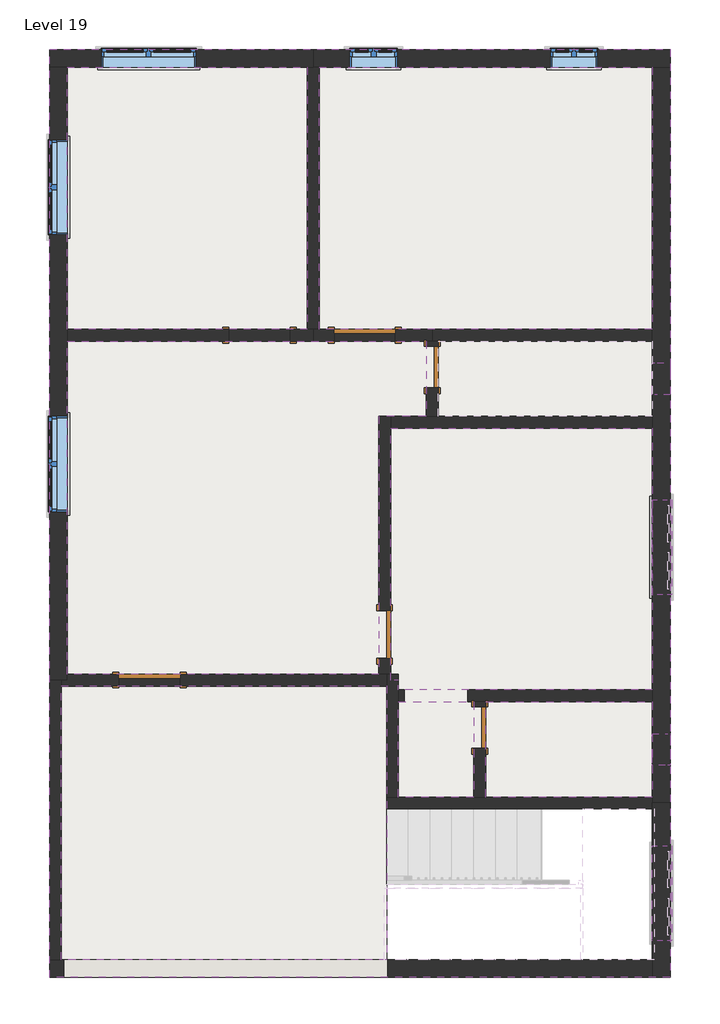
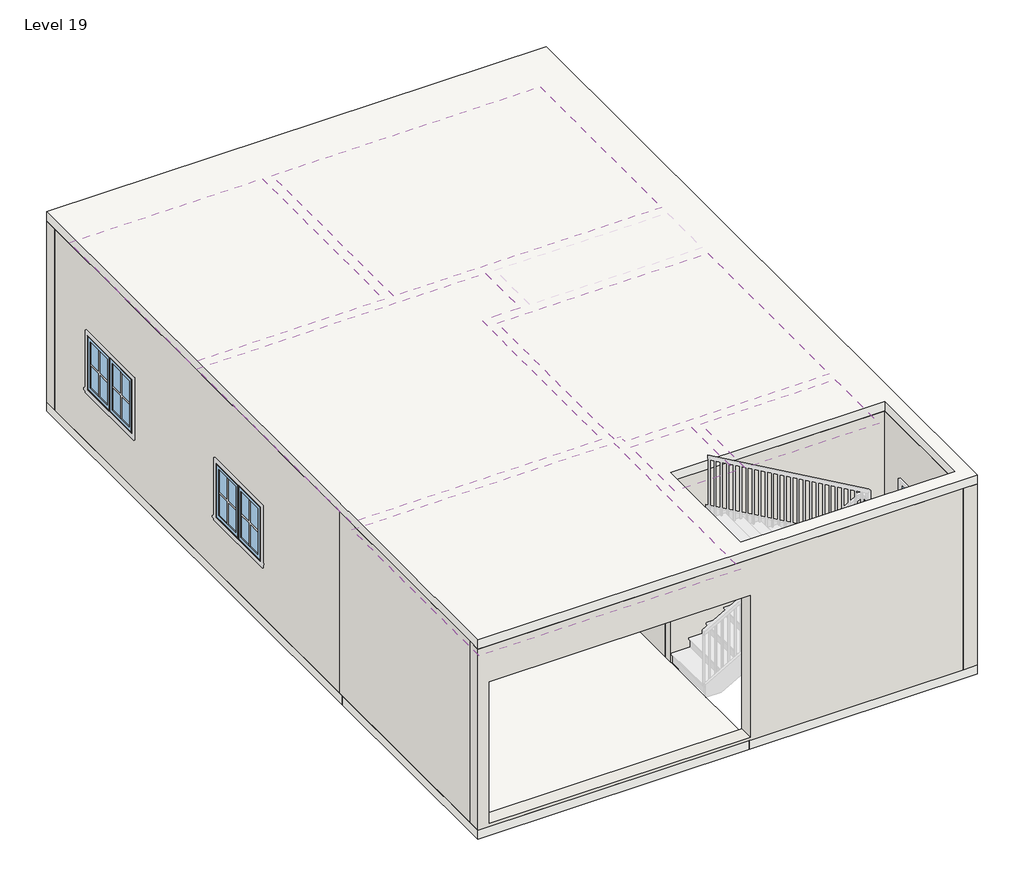
# One storey, part 1 of 2: 27 walls, 13 windows, 7 coverings, 6 doors, 3 slabs.
"""IFC4 building model written with IfcOpenShell, lengths in millimetres."""

from ifc_helpers import new_model, si_unit, frame, origin, place, context, project, spatial, polyline, outline, extrude, faceted_brep, transform, mapped, element, save
from components import door_2908be75, door_9ea4ff49, door_dc34e247, door_b804d09e, fixed_2_415b3208, window_casement_double_3_c417fced, window_casement_double_4_c19c33cb

model = new_model("IFC4")

# Units and contexts
model_context = context("Model", 3, world=origin())
ifc_project = project(units=[si_unit("LENGTHUNIT", "METRE", prefix="MILLI")], contexts=[model_context])

# Site, building, storey
site = spatial("IfcSite", under=ifc_project)
building = spatial("IfcBuilding", under=site)
storey = spatial("IfcBuildingStorey", under=building, Name="Level 19", Elevation=12801.6)

# Coverings
placement = place(None, origin())
element("IfcCovering", 1, ObjectType="2' x 4' ACT System", at=placement, inside=storey, context=model_context, shape_type="SweptSolid", body=[
    extrude(outline(polyline([(-5680.5154463, 2323.8455275), (-5680.5154463, 5678.2330275), (-2607.1154463, 5678.2330275), (-2607.1154463, 2323.8455275), (-5680.5154463, 2323.8455275)])), frame((0.0, 0.0, 15544.8), z_axis=(0.0, 0.0, 1.0), x_axis=(1.0, 0.0, 0.0)), (0.0, 0.0, 1.0), 57.15),
])
element("IfcCovering", 2, ObjectType="2' x 4' ACT System", at=placement, inside=storey, context=model_context, shape_type="SweptSolid", body=[
    extrude(outline(polyline([(-2454.7154463, 2323.8455275), (-2454.7154463, 5678.2330275), (1812.4845537, 5678.2330275), (1812.4845537, 2323.8455275), (-2454.7154463, 2323.8455275)])), frame((0.0, 0.0, 15544.8), z_axis=(0.0, 0.0, 1.0), x_axis=(1.0, 0.0, 0.0)), (0.0, 0.0, 1.0), 57.15),
])
element("IfcCovering", 3, ObjectType="2' x 4' ACT System", at=placement, inside=storey, context=model_context, shape_type="SweptSolid", body=[
    extrude(outline(polyline([(-5680.5154463, -2095.7544725), (-5680.5154463, 2171.4455275), (-1083.1154463, 2171.4455275), (-1083.1154463, 1206.2455275), (-1692.7154463, 1206.2455275), (-1692.7154463, -2095.7544725), (-5680.5154463, -2095.7544725)])), frame((0.0, 0.0, 15544.8), z_axis=(0.0, 0.0, 1.0), x_axis=(1.0, 0.0, 0.0)), (0.0, 0.0, 1.0), 57.15),
])
element("IfcCovering", 4, ObjectType="2' x 4' ACT System", at=placement, inside=storey, context=model_context, shape_type="SweptSolid", body=[
    extrude(outline(polyline([(1812.4845537, 1053.8455275), (1812.4845537, -2298.9544725), (-1438.7154463, -2298.9544725), (-1438.7154463, -2171.9544725), (-1540.3154463, -2171.9544725), (-1540.3154463, 1053.8455275), (1812.4845537, 1053.8455275)])), frame((0.0, 0.0, 15544.8), z_axis=(0.0, 0.0, 1.0), x_axis=(1.0, 0.0, 0.0)), (0.0, 0.0, 1.0), 57.15),
])
element("IfcCovering", 5, ObjectType="2' x 4' ACT System", at=placement, inside=storey, context=model_context, shape_type="SweptSolid", body=[
    extrude(outline(polyline([(1812.4845537, -2451.3544725), (1812.4845537, -3670.5544725), (-321.1154463, -3670.5544725), (-321.1154463, -2451.3544725), (1812.4845537, -2451.3544725)])), frame((0.0, 0.0, 15544.8), z_axis=(0.0, 0.0, 1.0), x_axis=(1.0, 0.0, 0.0)), (0.0, 0.0, 1.0), 57.15),
])
element("IfcCovering", 6, ObjectType="2' x 4' ACT System", at=placement, inside=storey, context=model_context, shape_type="SweptSolid", body=[
    extrude(outline(polyline([(-473.5154463, -2451.3544725), (-473.5154463, -3670.5544725), (-1438.7154463, -3670.5544725), (-1438.7154463, -2451.3544725), (-473.5154463, -2451.3544725)])), frame((0.0, 0.0, 15544.8), z_axis=(0.0, 0.0, 1.0), x_axis=(1.0, 0.0, 0.0)), (0.0, 0.0, 1.0), 57.15),
])
element("IfcCovering", 7, ObjectType="2' x 4' ACT System", at=placement, inside=storey, context=model_context, shape_type="SweptSolid", body=[
    extrude(outline(polyline([(-1591.1154463, -2248.1544725), (-1591.1154463, -5753.3544725), (-5756.7154463, -5753.3544725), (-5756.7154463, -2248.1544725), (-1591.1154463, -2248.1544725)])), frame((0.0, 0.0, 15544.8), z_axis=(0.0, 0.0, 1.0), x_axis=(1.0, 0.0, 0.0)), (0.0, 0.0, 1.0), 57.15),
])

# Doors
door_shape = door_2908be75(model_context)
element("IfcDoor", 8, ObjectType="Single-Flush : 1' 9\"", at=placement, inside=storey, context=model_context, shape_type="MappedRepresentation", body=[
    mapped(door_shape, transform((-397.3154463, -2781.5544725, 12801.6), x_axis=(0.0, 1.0, 0.0), y_axis=(-1.0, 0.0, 0.0), z_axis=(0.0, 0.0, 1.0))),
])
element("IfcDoor", 9, ObjectType="Single-Flush : 1' 9\"", at=placement, inside=storey, context=model_context, shape_type="MappedRepresentation", body=[
    mapped(door_shape, transform((-1006.9154463, 1841.2455275, 12801.6), x_axis=(0.0, 1.0, 0.0), y_axis=(-1.0, 0.0, 0.0), z_axis=(0.0, 0.0, 1.0))),
])
door_2_shape = door_9ea4ff49(model_context)
element("IfcDoor", 10, ObjectType="Single-Flush : 2'0\"", at=placement, inside=storey, context=model_context, shape_type="MappedRepresentation", body=[
    mapped(door_2_shape, transform((-1616.5154463, -1587.7544725, 12801.6), x_axis=(0.0, -1.0, 0.0), y_axis=(1.0, 0.0, 0.0), z_axis=(0.0, 0.0, 1.0))),
])
door_3_shape = door_dc34e247(model_context)
element("IfcDoor", 11, ObjectType="Single-Flush : 2'7\"", at=placement, inside=storey, context=model_context, shape_type="MappedRepresentation", body=[
    mapped(door_3_shape, transform((-4626.4154463, -2171.9544725, 12801.6), x_axis=(-1.0, 0.0, 0.0), y_axis=(0.0, -1.0, 0.0), z_axis=(0.0, 0.0, 1.0))),
])
element("IfcDoor", 12, ObjectType="Single-Flush : 2'7\"", at=placement, inside=storey, context=model_context, shape_type="MappedRepresentation", body=[
    mapped(door_3_shape, transform((-1870.5154463, 2247.6455275, 12801.6), x_axis=(-1.0, 0.0, 0.0), y_axis=(0.0, -1.0, 0.0), z_axis=(0.0, 0.0, 1.0))),
])
door_4_shape = door_b804d09e(model_context)
element("IfcDoor", 13, ObjectType="Single-Flush : 2'7\"", at=placement, inside=storey, context=model_context, shape_type="MappedRepresentation", body=[
    mapped(door_4_shape, transform((-3216.7154463, 2247.6455275, 12801.6), x_axis=(1.0, 0.0, 0.0), y_axis=(0.0, 1.0, 0.0), z_axis=(0.0, 0.0, 1.0))),
])

# Slabs
element("IfcSlab", 14, ObjectType="Generic - 6\"", at=placement, inside=storey, context=model_context, shape_type="SweptSolid", body=[
    extrude(outline(polyline([(-5909.1154463, -2248.1544725), (-5909.1154463, 5906.8330275), (2041.0845537, 5906.8330275), (2041.0845537, -5981.9544725), (-1591.1154463, -5981.9544725), (-1591.1154463, -5753.3544725), (1812.4845537, -5753.3544725), (1812.4845537, -3822.9544725), (-1591.1154463, -3822.9544725), (-1591.1154463, -2248.1544725), (-5756.7154463, -2248.1544725), (-5909.1154463, -2248.1544725)])), frame((0.0, 0.0, 12649.2), z_axis=(0.0, 0.0, 1.0), x_axis=(1.0, 0.0, 0.0)), (0.0, 0.0, 1.0), 152.4),
])
element("IfcSlab", 15, ObjectType="Generic - 6\"", at=placement, inside=storey, context=model_context, shape_type="SweptSolid", body=[
    extrude(outline(polyline([(-1591.1154463, -2248.1544725), (-1591.1154463, -5981.9544725), (-5909.1154463, -5981.9544725), (-5909.1154463, -2248.1544725), (-1591.1154463, -2248.1544725)])), frame((0.0, 0.0, 12649.2), z_axis=(0.0, 0.0, 1.0), x_axis=(1.0, 0.0, 0.0)), (0.0, 0.0, 1.0), 152.4),
])
element("IfcSlab", 16, ObjectType="Generic - 6\"", at=placement, inside=storey, context=model_context, shape_type="SweptSolid", body=[
    extrude(outline(polyline([(2041.0845537, 5906.8330275), (2041.0845537, -5981.9544725), (-5909.1154463, -5981.9544725), (-5909.1154463, 5906.8330275), (2041.0845537, 5906.8330275)]), holes=[polyline([(1812.4845537, -3822.9544725), (-1591.1154463, -3822.9544725), (-1591.1154463, -5753.3544725), (1812.4845537, -5753.3544725), (1812.4845537, -3822.9544725)])]), frame((0.0, 0.0, 15849.6), z_axis=(0.0, 0.0, 1.0), x_axis=(1.0, 0.0, 0.0)), (0.0, 0.0, 1.0), 152.4),
])

# Walls
element("IfcWall", 17, ObjectType="Generic - 6\"", at=placement, inside=storey, context=model_context, shape_type="Brep", body=[
    faceted_brep([(-5909.1154463, -2171.9544725, 12801.6), (-5909.1154463, -5753.3544725, 12801.6), (-5909.1154463, -5753.3544725, 15849.6), (-5909.1154463, -2171.9544725, 15849.6), (-5756.7154463, -2171.9544725, 12801.6), (-5756.7154463, -2171.9544725, 15849.6), (-5756.7154463, -2248.1544725, 15849.6), (-5756.7154463, -5753.3544725, 15849.6), (-5756.7154463, -5753.3544725, 12801.6), (-5756.7154463, -2248.1544725, 12801.6)], [[[0, 1, 2, 3]], [[4, 5, 6, 7, 8, 9]], [[1, 0, 4, 9, 8]], [[3, 2, 7, 6, 5]], [[0, 3, 5, 4]], [[2, 1, 8, 7]]]),
])
element("IfcWall", 18, ObjectType="Generic - 6\"", at=placement, inside=storey, context=model_context, shape_type="Brep", body=[
    faceted_brep([(1812.4845537, -3670.5544725, 12801.6), (-321.1154463, -3670.5544725, 12801.6), (-473.5154463, -3670.5544725, 12801.6), (-1438.7154463, -3670.5544725, 12801.6), (-1591.1154463, -3670.5544725, 12801.6), (-1591.1154463, -3670.5544725, 15849.6), (-1438.7154463, -3670.5544725, 15849.6), (-473.5154463, -3670.5544725, 15849.6), (-321.1154463, -3670.5544725, 15849.6), (1812.4845537, -3670.5544725, 15849.6), (1812.4845537, -3822.9544725, 12801.6), (1812.4845537, -3822.9544725, 15849.6), (-1591.1154463, -3822.9544725, 15849.6), (-1591.1154463, -3822.9544725, 12801.6), (1812.4845537, -3746.7544725, 12801.6), (1812.4845537, -3746.7544725, 15849.6)], [[[0, 1, 2, 3, 4, 5, 6, 7, 8, 9]], [[10, 11, 12, 13]], [[4, 3, 2, 1, 0, 14, 10, 13]], [[9, 8, 7, 6, 5, 12, 11, 15]], [[5, 4, 13, 12]], [[0, 9, 15, 11, 10, 14]]]),
])
element("IfcWall", 19, ObjectType="Generic - 6\"", at=placement, inside=storey, context=model_context, shape_type="Brep", body=[
    faceted_brep([(-1438.7154463, -3670.5544725, 12801.6), (-1438.7154463, -2451.3544725, 12801.6), (-1438.7154463, -2298.9544725, 12801.6), (-1438.7154463, -2095.7544725, 12801.6), (-1438.7154463, -2095.7544725, 15849.6), (-1438.7154463, -2298.9544725, 15849.6), (-1438.7154463, -2451.3544725, 15849.6), (-1438.7154463, -3670.5544725, 15849.6), (-1591.1154463, -3670.5544725, 12801.6), (-1591.1154463, -3670.5544725, 15849.6), (-1591.1154463, -2248.1544725, 15849.6), (-1591.1154463, -2171.9544725, 15849.6), (-1591.1154463, -2095.7544725, 15849.6), (-1591.1154463, -2095.7544725, 12801.6), (-1591.1154463, -2171.9544725, 12801.6), (-1591.1154463, -2248.1544725, 12801.6), (-1540.3154463, -2095.7544725, 12801.6), (-1540.3154463, -2095.7544725, 15849.6)], [[[0, 1, 2, 3, 4, 5, 6, 7]], [[8, 9, 10, 11, 12, 13, 14, 15]], [[3, 2, 1, 0, 8, 15, 14, 13, 16]], [[7, 6, 5, 4, 17, 12, 11, 10, 9]], [[0, 7, 9, 8]], [[4, 3, 16, 13, 12, 17]]]),
])
element("IfcWall", 20, ObjectType="Generic - 6\"", at=placement, inside=storey, context=model_context, shape_type="Brep", body=[
    faceted_brep([(-5020.1154463, -2095.7544725, 14935.2), (-5020.1154463, -2095.7544725, 12801.6), (-5680.5154463, -2095.7544725, 12801.6), (-5680.5154463, -2095.7544725, 15849.6), (-1692.7154463, -2095.7544725, 15849.6), (-1591.1154463, -2095.7544725, 15849.6), (-1591.1154463, -2095.7544725, 12801.6), (-1692.7154463, -2095.7544725, 12801.6), (-4232.7154463, -2095.7544725, 12801.6), (-4232.7154463, -2095.7544725, 14935.2), (-5756.7154463, -2248.1544725, 12801.6), (-5020.1154463, -2248.1544725, 12801.6), (-5020.1154463, -2248.1544725, 14935.2), (-4232.7154463, -2248.1544725, 14935.2), (-4232.7154463, -2248.1544725, 12801.6), (-1591.1154463, -2248.1544725, 12801.6), (-1591.1154463, -2248.1544725, 15849.6), (-5756.7154463, -2248.1544725, 15849.6), (-5756.7154463, -2171.9544725, 12801.6), (-5680.5154463, -2171.9544725, 12801.6), (-5680.5154463, -2171.9544725, 15849.6), (-5756.7154463, -2171.9544725, 15849.6)], [[[0, 1, 2, 3, 4, 5, 6, 7, 8, 9]], [[10, 11, 12, 13, 14, 15, 16, 17]], [[2, 1, 11, 10, 18, 19]], [[8, 7, 6, 15, 14]], [[5, 4, 3, 20, 21, 17, 16]], [[3, 2, 19, 20]], [[19, 18, 21, 20]], [[18, 10, 17, 21]], [[6, 5, 16, 15]], [[12, 11, 1, 0]], [[13, 12, 0, 9]], [[14, 13, 9, 8]]]),
])
element("IfcWall", 21, ObjectType="Generic - 6\"", at=placement, inside=storey, context=model_context, shape_type="Brep", body=[
    faceted_brep([(1812.4845537, -2451.3544725, 12801.6), (1812.4845537, -2451.3544725, 15849.6), (-321.1154463, -2451.3544725, 15849.6), (-473.5154463, -2451.3544725, 15849.6), (-1438.7154463, -2451.3544725, 15849.6), (-1438.7154463, -2451.3544725, 12801.6), (-1367.0206652, -2451.3544725, 12801.6), (-1367.0206652, -2451.3544725, 15240.0), (-547.4818767, -2451.3544725, 15240.0), (-547.4818767, -2451.3544725, 12801.6), (-473.5154463, -2451.3544725, 12801.6), (-321.1154463, -2451.3544725, 12801.6), (1812.4845537, -2298.9544725, 15849.6), (1812.4845537, -2298.9544725, 12801.6), (-547.4818767, -2298.9544725, 12801.6), (-547.4818767, -2298.9544725, 15240.0), (-1367.0206652, -2298.9544725, 15240.0), (-1367.0206652, -2298.9544725, 12801.6), (-1438.7154463, -2298.9544725, 12801.6), (-1438.7154463, -2298.9544725, 15849.6)], [[[0, 1, 2, 3, 4, 5, 6, 7, 8, 9, 10, 11]], [[12, 13, 14, 15, 16, 17, 18, 19]], [[5, 18, 17, 6]], [[13, 0, 11, 10, 9, 14]], [[4, 3, 2, 1, 12, 19]], [[1, 0, 13, 12]], [[5, 4, 19, 18]], [[7, 16, 15, 8]], [[16, 7, 6, 17]], [[8, 15, 14, 9]]]),
])
element("IfcWall", 22, ObjectType="Generic - 6\"", at=placement, inside=storey, context=model_context, shape_type="SweptSolid", body=[
    extrude(outline(polyline([(-2451.3544725, 12801.6), (-2514.8544725, 12801.6), (-2514.8544725, 14935.2), (-3048.2544725, 14935.2), (-3048.2544725, 12801.6), (-3670.5544725, 12801.6), (-3670.5544725, 15849.6), (-2451.3544725, 15849.6), (-2451.3544725, 12801.6)])), frame((-473.5154463, 0.0, 0.0), z_axis=(1.0, 0.0, 0.0), x_axis=(0.0, 1.0, 0.0)), (0.0, 0.0, 1.0), 152.4),
])
element("IfcWall", 23, ObjectType="Generic - 6\"", at=placement, inside=storey, context=model_context, shape_type="Brep", body=[
    faceted_brep([(-1540.3154463, -2095.7544725, 12801.6), (-1540.3154463, -1892.5544725, 12801.6), (-1540.3154463, -1892.5544725, 14935.2), (-1540.3154463, -1282.9544725, 14935.2), (-1540.3154463, -1282.9544725, 12801.6), (-1540.3154463, 1053.8455275, 12801.6), (-1540.3154463, 1206.2455275, 12801.6), (-1540.3154463, 1206.2455275, 15849.6), (-1540.3154463, 1053.8455275, 15849.6), (-1540.3154463, -2095.7544725, 15849.6), (-1692.7154463, -1892.5544725, 14935.2), (-1692.7154463, -1892.5544725, 12801.6), (-1692.7154463, -2095.7544725, 12801.6), (-1692.7154463, -2095.7544725, 15849.6), (-1692.7154463, 1206.2455275, 15849.6), (-1692.7154463, 1206.2455275, 12801.6), (-1692.7154463, -1282.9544725, 12801.6), (-1692.7154463, -1282.9544725, 14935.2), (-1591.1154463, -2095.7544725, 12801.6), (-1591.1154463, -2095.7544725, 15849.6)], [[[0, 1, 2, 3, 4, 5, 6, 7, 8, 9]], [[10, 11, 12, 13, 14, 15, 16, 17]], [[16, 15, 6, 5, 4]], [[12, 11, 1, 0, 18]], [[9, 8, 7, 14, 13, 19]], [[0, 9, 19, 13, 12, 18]], [[7, 6, 15, 14]], [[2, 1, 11, 10]], [[3, 2, 10, 17]], [[4, 3, 17, 16]]]),
])
element("IfcWall", 24, ObjectType="Generic - 6\"", at=placement, inside=storey, context=model_context, shape_type="Brep", body=[
    faceted_brep([(-1540.3154463, 1053.8455275, 12801.6), (1812.4845537, 1053.8455275, 12801.6), (1812.4845537, 1053.8455275, 15849.6), (-1540.3154463, 1053.8455275, 15849.6), (-1540.3154463, 1206.2455275, 12801.6), (-1540.3154463, 1206.2455275, 15849.6), (-1083.1154463, 1206.2455275, 15849.6), (-930.7154463, 1206.2455275, 15849.6), (1812.4845537, 1206.2455275, 15849.6), (1812.4845537, 1206.2455275, 12801.6), (-930.7154463, 1206.2455275, 12801.6), (-1083.1154463, 1206.2455275, 12801.6)], [[[0, 1, 2, 3]], [[4, 5, 6, 7, 8, 9, 10, 11]], [[1, 0, 4, 11, 10, 9]], [[3, 2, 8, 7, 6, 5]], [[0, 3, 5, 4]], [[2, 1, 9, 8]]]),
])
element("IfcWall", 25, ObjectType="Generic - 6\"", at=placement, inside=storey, context=model_context, shape_type="Brep", body=[
    faceted_brep([(-930.7154463, 2107.9455275, 14935.2), (-930.7154463, 2107.9455275, 12801.6), (-930.7154463, 2171.4455275, 12801.6), (-930.7154463, 2171.4455275, 15849.6), (-930.7154463, 1206.2455275, 15849.6), (-930.7154463, 1206.2455275, 12801.6), (-930.7154463, 1574.5455275, 12801.6), (-930.7154463, 1574.5455275, 14935.2), (-1083.1154463, 2171.4455275, 12801.6), (-1083.1154463, 2107.9455275, 12801.6), (-1083.1154463, 2107.9455275, 14935.2), (-1083.1154463, 1574.5455275, 14935.2), (-1083.1154463, 1574.5455275, 12801.6), (-1083.1154463, 1206.2455275, 12801.6), (-1083.1154463, 1206.2455275, 15849.6), (-1083.1154463, 2171.4455275, 15849.6), (-1006.9154463, 2171.4455275, 12801.6), (-1006.9154463, 2171.4455275, 15849.6)], [[[0, 1, 2, 3, 4, 5, 6, 7]], [[8, 9, 10, 11, 12, 13, 14, 15]], [[6, 5, 13, 12]], [[2, 1, 9, 8, 16]], [[4, 3, 17, 15, 14]], [[5, 4, 14, 13]], [[10, 9, 1, 0]], [[11, 10, 0, 7]], [[12, 11, 7, 6]], [[3, 2, 16, 8, 15, 17]]]),
])
element("IfcWall", 26, ObjectType="Generic - 6\"", at=placement, inside=storey, context=model_context, shape_type="Brep", body=[
    faceted_brep([(1812.4845537, 2323.8455275, 12801.6), (-1006.9154463, 2323.8455275, 12801.6), (-1006.9154463, 2323.8455275, 15849.6), (1812.4845537, 2323.8455275, 15849.6), (1812.4845537, 2171.4455275, 12801.6), (1812.4845537, 2171.4455275, 15849.6), (-930.7154463, 2171.4455275, 15849.6), (-1006.9154463, 2171.4455275, 15849.6), (-1006.9154463, 2171.4455275, 12801.6), (-930.7154463, 2171.4455275, 12801.6)], [[[0, 1, 2, 3]], [[4, 5, 6, 7, 8, 9]], [[1, 0, 4, 9, 8]], [[2, 1, 8, 7]], [[3, 2, 7, 6, 5]], [[0, 3, 5, 4]]]),
])
element("IfcWall", 27, ObjectType="Generic - 6\"", at=placement, inside=storey, context=model_context, shape_type="Brep", body=[
    faceted_brep([(-2607.1154463, 5678.2330275, 12801.6), (-2607.1154463, 2323.8455275, 12801.6), (-2607.1154463, 2323.8455275, 15849.6), (-2607.1154463, 5678.2330275, 15849.6), (-2454.7154463, 5678.2330275, 12801.6), (-2454.7154463, 5678.2330275, 15849.6), (-2454.7154463, 2323.8455275, 15849.6), (-2454.7154463, 2323.8455275, 12801.6), (-2530.9154463, 5678.2330275, 12801.6), (-2530.9154463, 2323.8455275, 12801.6), (-2530.9154463, 2323.8455275, 15849.6), (-2530.9154463, 5678.2330275, 15849.6)], [[[0, 1, 2, 3]], [[4, 5, 6, 7]], [[1, 0, 8, 4, 7, 9]], [[3, 2, 10, 6, 5, 11]], [[0, 3, 11, 5, 4, 8]], [[2, 1, 9, 7, 6, 10]]]),
])
element("IfcWall", 28, ObjectType="Generic - 6\"", at=placement, inside=storey, context=model_context, shape_type="Brep", body=[
    faceted_brep([(-2530.9154463, 2323.8455275, 12801.6), (-2607.1154463, 2323.8455275, 12801.6), (-2823.0154463, 2323.8455275, 12801.6), (-2823.0154463, 2323.8455275, 14935.2), (-3610.4154463, 2323.8455275, 14935.2), (-3610.4154463, 2323.8455275, 12801.6), (-5680.5154463, 2323.8455275, 12801.6), (-5680.5154463, 2323.8455275, 15849.6), (-2607.1154463, 2323.8455275, 15849.6), (-2530.9154463, 2323.8455275, 15849.6), (-2823.0154463, 2171.4455275, 14935.2), (-2823.0154463, 2171.4455275, 12801.6), (-2530.9154463, 2171.4455275, 12801.6), (-2530.9154463, 2171.4455275, 15849.6), (-5680.5154463, 2171.4455275, 15849.6), (-5680.5154463, 2171.4455275, 12801.6), (-3610.4154463, 2171.4455275, 12801.6), (-3610.4154463, 2171.4455275, 14935.2)], [[[0, 1, 2, 3, 4, 5, 6, 7, 8, 9]], [[10, 11, 12, 13, 14, 15, 16, 17]], [[16, 15, 6, 5]], [[12, 11, 2, 1, 0]], [[9, 8, 7, 14, 13]], [[0, 9, 13, 12]], [[7, 6, 15, 14]], [[5, 4, 17, 16]], [[4, 3, 10, 17]], [[3, 2, 11, 10]]]),
])
element("IfcWall", 29, ObjectType="Generic - 6\"", at=placement, inside=storey, context=model_context, shape_type="Brep", body=[
    faceted_brep([(-2264.2154463, 2323.8455275, 14935.2), (-2264.2154463, 2323.8455275, 12801.6), (-2454.7154463, 2323.8455275, 12801.6), (-2530.9154463, 2323.8455275, 12801.6), (-2530.9154463, 2323.8455275, 15849.6), (-2454.7154463, 2323.8455275, 15849.6), (-1006.9154463, 2323.8455275, 15849.6), (-1006.9154463, 2323.8455275, 12801.6), (-1476.8154463, 2323.8455275, 12801.6), (-1476.8154463, 2323.8455275, 14935.2), (-2530.9154463, 2171.4455275, 12801.6), (-2264.2154463, 2171.4455275, 12801.6), (-2264.2154463, 2171.4455275, 14935.2), (-1476.8154463, 2171.4455275, 14935.2), (-1476.8154463, 2171.4455275, 12801.6), (-1083.1154463, 2171.4455275, 12801.6), (-1006.9154463, 2171.4455275, 12801.6), (-1006.9154463, 2171.4455275, 15849.6), (-1083.1154463, 2171.4455275, 15849.6), (-2530.9154463, 2171.4455275, 15849.6)], [[[0, 1, 2, 3, 4, 5, 6, 7, 8, 9]], [[10, 11, 12, 13, 14, 15, 16, 17, 18, 19]], [[8, 7, 16, 15, 14]], [[3, 2, 1, 11, 10]], [[4, 3, 10, 19]], [[6, 5, 4, 19, 18, 17]], [[7, 6, 17, 16]], [[14, 13, 9, 8]], [[13, 12, 0, 9]], [[12, 11, 1, 0]]]),
])
element("IfcWall", 30, ObjectType="Generic - 6\"", at=placement, inside=storey, context=model_context, shape_type="SweptSolid", body=[
    extrude(outline(polyline([(-5680.5154463, -2095.7544725), (-1692.7154463, -2095.7544725), (-1692.7154463, -2171.9544725), (-1591.1154463, -2171.9544725), (-1591.1154463, -2248.1544725), (-5756.7154463, -2248.1544725), (-5756.7154463, -2171.9544725), (-5680.5154463, -2171.9544725), (-5680.5154463, -2095.7544725)])), frame((0.0, 0.0, 12801.6), z_axis=(0.0, 0.0, 1.0), x_axis=(1.0, 0.0, 0.0)), (0.0, 0.0, 1.0), 3048.0),
])
element("IfcWall", 31, ObjectType="Generic - 6\"", at=placement, inside=storey, context=model_context, shape_type="Brep", body=[
    faceted_brep([(-2607.1154463, 5678.2330275, 12801.6), (-2607.1154463, 2323.8455275, 12801.6), (-2607.1154463, 2323.8455275, 15849.6), (-2607.1154463, 5678.2330275, 15849.6), (-2454.7154463, 5678.2330275, 12801.6), (-2454.7154463, 5678.2330275, 15849.6), (-2454.7154463, 2323.8455275, 15849.6), (-2454.7154463, 2323.8455275, 12801.6), (-2530.9154463, 5678.2330275, 12801.6), (-2530.9154463, 2323.8455275, 12801.6), (-2530.9154463, 2323.8455275, 15849.6), (-2530.9154463, 5678.2330275, 15849.6)], [[[0, 1, 2, 3]], [[4, 5, 6, 7]], [[1, 0, 8, 4, 7, 9]], [[3, 2, 10, 6, 5, 11]], [[0, 3, 11, 5, 4, 8]], [[2, 1, 9, 7, 6, 10]]]),
])
element("IfcWall", 32, ObjectType="Generic - 6\"", at=placement, inside=storey, context=model_context, shape_type="Brep", body=[
    faceted_brep([(-2530.9154463, 2323.8455275, 12801.6), (-2607.1154463, 2323.8455275, 12801.6), (-5680.5154463, 2323.8455275, 12801.6), (-5680.5154463, 2323.8455275, 15849.6), (-2607.1154463, 2323.8455275, 15849.6), (-2530.9154463, 2323.8455275, 15849.6), (-2530.9154463, 2171.4455275, 12801.6), (-2530.9154463, 2171.4455275, 15849.6), (-5680.5154463, 2171.4455275, 15849.6), (-5680.5154463, 2171.4455275, 12801.6)], [[[0, 1, 2, 3, 4, 5]], [[6, 7, 8, 9]], [[2, 1, 0, 6, 9]], [[5, 4, 3, 8, 7]], [[0, 5, 7, 6]], [[3, 2, 9, 8]]]),
])
element("IfcWall", 33, ObjectType="Generic - 6\"", at=placement, inside=storey, context=model_context, shape_type="Brep", body=[
    faceted_brep([(-1006.9154463, 2323.8455275, 12801.6), (-2454.7154463, 2323.8455275, 12801.6), (-2530.9154463, 2323.8455275, 12801.6), (-2530.9154463, 2323.8455275, 15849.6), (-2454.7154463, 2323.8455275, 15849.6), (-1006.9154463, 2323.8455275, 15849.6), (-1006.9154463, 2171.4455275, 12801.6), (-1006.9154463, 2171.4455275, 15849.6), (-1083.1154463, 2171.4455275, 15849.6), (-2530.9154463, 2171.4455275, 15849.6), (-2530.9154463, 2171.4455275, 12801.6), (-1083.1154463, 2171.4455275, 12801.6)], [[[0, 1, 2, 3, 4, 5]], [[6, 7, 8, 9, 10, 11]], [[2, 1, 0, 6, 11, 10]], [[3, 2, 10, 9]], [[5, 4, 3, 9, 8, 7]], [[0, 5, 7, 6]]]),
])
element("IfcWall", 34, ObjectType="Generic - 9\"", at=placement, inside=storey, context=model_context, shape_type="Brep", body=[
    faceted_brep([(-5909.1154463, 5678.2330275, 12801.6), (-5680.5154463, 5678.2330275, 12801.6), (-2607.1154463, 5678.2330275, 12801.6), (-2530.9154463, 5678.2330275, 12801.6), (-2530.9154463, 5678.2330275, 15849.6), (-2607.1154463, 5678.2330275, 15849.6), (-5680.5154463, 5678.2330275, 15849.6), (-5909.1154463, 5678.2330275, 15849.6), (-4029.5154463, 5678.2330275, 14630.4), (-4029.5154463, 5678.2330275, 13716.0), (-5248.7154463, 5678.2330275, 13716.0), (-5248.7154463, 5678.2330275, 14630.4), (-5909.1154463, 5906.8330275, 12801.6), (-5909.1154463, 5906.8330275, 15849.6), (-2530.9154463, 5906.8330275, 15849.6), (-2530.9154463, 5906.8330275, 12801.6), (-4029.5154463, 5906.8330275, 14630.4), (-5248.7154463, 5906.8330275, 14630.4), (-5248.7154463, 5906.8330275, 13716.0), (-4029.5154463, 5906.8330275, 13716.0)], [[[0, 1, 2, 3, 4, 5, 6, 7], [8, 9, 10, 11]], [[12, 13, 14, 15], [16, 17, 18, 19]], [[3, 2, 1, 0, 12, 15]], [[4, 3, 15, 14]], [[7, 6, 5, 4, 14, 13]], [[0, 7, 13, 12]], [[9, 8, 16, 19]], [[10, 9, 19, 18]], [[11, 10, 18, 17]], [[8, 11, 17, 16]]]),
])
element("IfcWall", 35, ObjectType="Generic - 9\"", at=placement, inside=storey, context=model_context, shape_type="Brep", body=[
    faceted_brep([(1812.4845537, 5678.2330275, 12801.6), (1812.4845537, 2323.8455275, 12801.6), (1812.4845537, 2171.4455275, 12801.6), (1812.4845537, 1206.2455275, 12801.6), (1812.4845537, 1053.8455275, 12801.6), (1812.4845537, -2298.9544725, 12801.6), (1812.4845537, -2451.3544725, 12801.6), (1812.4845537, -3670.5544725, 12801.6), (1812.4845537, -3746.7544725, 12801.6), (1812.4845537, -3746.7544725, 15849.6), (1812.4845537, -3670.5544725, 15849.6), (1812.4845537, -2451.3544725, 15849.6), (1812.4845537, -2298.9544725, 15849.6), (1812.4845537, 1053.8455275, 15849.6), (1812.4845537, 1206.2455275, 15849.6), (1812.4845537, 2171.4455275, 15849.6), (1812.4845537, 2323.8455275, 15849.6), (1812.4845537, 5678.2330275, 15849.6), (1812.4845537, -1079.7544725, 14935.2), (1812.4845537, -1079.7544725, 14020.8), (1812.4845537, 139.4455275, 14020.8), (1812.4845537, 139.4455275, 14935.2), (1812.4845537, -3264.1544725, 15240.0), (1812.4845537, -3264.1544725, 14630.4), (1812.4845537, -2857.7544725, 14630.4), (1812.4845537, -2857.7544725, 15240.0), (1812.4845537, 1892.0455275, 15240.0), (1812.4845537, 1485.6455275, 15240.0), (1812.4845537, 1485.6455275, 14630.4), (1812.4845537, 1892.0455275, 14630.4), (2041.0845537, 5678.2330275, 12801.6), (2041.0845537, 5678.2330275, 15849.6), (2041.0845537, -3746.7544725, 15849.6), (2041.0845537, -3746.7544725, 12801.6), (2041.0845537, -1079.7544725, 14935.2), (2041.0845537, 139.4455275, 14935.2), (2041.0845537, 139.4455275, 14020.8), (2041.0845537, -1079.7544725, 14020.8), (2041.0845537, -3264.1544725, 15240.0), (2041.0845537, -2857.7544725, 15240.0), (2041.0845537, -2857.7544725, 14630.4), (2041.0845537, -3264.1544725, 14630.4), (2041.0845537, 1892.0455275, 15240.0), (2041.0845537, 1892.0455275, 14630.4), (2041.0845537, 1485.6455275, 14630.4), (2041.0845537, 1485.6455275, 15240.0)], [[[0, 1, 2, 3, 4, 5, 6, 7, 8, 9, 10, 11, 12, 13, 14, 15, 16, 17], [18, 19, 20, 21], [22, 23, 24, 25], [26, 27, 28, 29]], [[30, 31, 32, 33], [34, 35, 36, 37], [38, 39, 40, 41], [42, 43, 44, 45]], [[8, 7, 6, 5, 4, 3, 2, 1, 0, 30, 33]], [[9, 8, 33, 32]], [[17, 16, 15, 14, 13, 12, 11, 10, 9, 32, 31]], [[0, 17, 31, 30]], [[19, 18, 34, 37]], [[20, 19, 37, 36]], [[21, 20, 36, 35]], [[18, 21, 35, 34]], [[23, 22, 38, 41]], [[24, 23, 41, 40]], [[25, 24, 40, 39]], [[22, 25, 39, 38]], [[43, 42, 26, 29]], [[44, 43, 29, 28]], [[45, 44, 28, 27]], [[42, 45, 27, 26]]]),
])
element("IfcWall", 36, ObjectType="Generic - 9\"", at=placement, inside=storey, context=model_context, shape_type="Brep", body=[
    faceted_brep([(1812.4845537, -5753.3544725, 12801.6), (-5756.7154463, -5753.3544725, 12801.6), (-5909.1154463, -5753.3544725, 12801.6), (-5909.1154463, -5753.3544725, 15849.6), (-5756.7154463, -5753.3544725, 15849.6), (1812.4845537, -5753.3544725, 15849.6), (-1576.8982041, -5753.3544725, 15240.0), (-5729.1673724, -5753.3544725, 15240.0), (-5729.1673724, -5753.3544725, 12852.4), (-1576.8982041, -5753.3544725, 12852.4), (-5909.1154463, -5981.9544725, 12801.6), (1812.4845537, -5981.9544725, 12801.6), (1812.4845537, -5981.9544725, 15849.6), (-5909.1154463, -5981.9544725, 15849.6), (-5729.1673724, -5981.9544725, 15240.0), (-1576.8982041, -5981.9544725, 15240.0), (-1576.8982041, -5981.9544725, 12852.4), (-5729.1673724, -5981.9544725, 12852.4)], [[[0, 1, 2, 3, 4, 5], [6, 7, 8, 9]], [[10, 11, 12, 13], [14, 15, 16, 17]], [[2, 1, 0, 11, 10]], [[5, 4, 3, 13, 12]], [[0, 5, 12, 11]], [[6, 15, 14, 7]], [[8, 17, 16, 9]], [[15, 6, 9, 16]], [[7, 14, 17, 8]], [[3, 2, 10, 13]]]),
])
element("IfcWall", 37, ObjectType="Generic - 9\"", at=placement, inside=storey, context=model_context, shape_type="Brep", body=[
    faceted_brep([(-5909.1154463, 5678.2330275, 12801.6), (-5909.1154463, -2171.9544725, 12801.6), (-5909.1154463, -2171.9544725, 15849.6), (-5909.1154463, 5678.2330275, 15849.6), (-5909.1154463, 4751.1330275, 14630.4), (-5909.1154463, 3531.9330275, 14630.4), (-5909.1154463, 3531.9330275, 13716.0), (-5909.1154463, 4751.1330275, 13716.0), (-5909.1154463, 1206.2455275, 14630.4), (-5909.1154463, -12.9544725, 14630.4), (-5909.1154463, -12.9544725, 13716.0), (-5909.1154463, 1206.2455275, 13716.0), (-5680.5154463, 5678.2330275, 12801.6), (-5680.5154463, 5678.2330275, 15849.6), (-5680.5154463, 2323.8455275, 15849.6), (-5680.5154463, 2171.4455275, 15849.6), (-5680.5154463, -2095.7544725, 15849.6), (-5680.5154463, -2171.9544725, 15849.6), (-5680.5154463, -2171.9544725, 12801.6), (-5680.5154463, -2095.7544725, 12801.6), (-5680.5154463, 2171.4455275, 12801.6), (-5680.5154463, 2323.8455275, 12801.6), (-5680.5154463, 4751.1330275, 14630.4), (-5680.5154463, 4751.1330275, 13716.0), (-5680.5154463, 3531.9330275, 13716.0), (-5680.5154463, 3531.9330275, 14630.4), (-5680.5154463, 1206.2455275, 14630.4), (-5680.5154463, 1206.2455275, 13716.0), (-5680.5154463, -12.9544725, 13716.0), (-5680.5154463, -12.9544725, 14630.4), (-5756.7154463, -2171.9544725, 12801.6), (-5756.7154463, -2171.9544725, 15849.6)], [[[0, 1, 2, 3], [4, 5, 6, 7], [8, 9, 10, 11]], [[12, 13, 14, 15, 16, 17, 18, 19, 20, 21], [22, 23, 24, 25], [26, 27, 28, 29]], [[1, 0, 12, 21, 20, 19, 18, 30]], [[2, 1, 30, 18, 17, 31]], [[3, 2, 31, 17, 16, 15, 14, 13]], [[0, 3, 13, 12]], [[23, 22, 4, 7]], [[24, 23, 7, 6]], [[25, 24, 6, 5]], [[22, 25, 5, 4]], [[27, 26, 8, 11]], [[28, 27, 11, 10]], [[29, 28, 10, 9]], [[26, 29, 9, 8]]]),
])
element("IfcWall", 38, ObjectType="Generic - 9\"", at=placement, inside=storey, context=model_context, shape_type="Brep", body=[
    faceted_brep([(-2530.9154463, 5678.2330275, 12801.6), (-2454.7154463, 5678.2330275, 12801.6), (1812.4845537, 5678.2330275, 12801.6), (2041.0845537, 5678.2330275, 12801.6), (2041.0845537, 5678.2330275, 15849.6), (1812.4845537, 5678.2330275, 15849.6), (-2454.7154463, 5678.2330275, 15849.6), (-2530.9154463, 5678.2330275, 15849.6), (-1451.4154463, 5678.2330275, 14630.4), (-1451.4154463, 5678.2330275, 13716.0), (-2061.0154463, 5678.2330275, 13716.0), (-2061.0154463, 5678.2330275, 14630.4), (1113.9845537, 5678.2330275, 14630.4), (1113.9845537, 5678.2330275, 13716.0), (504.3845537, 5678.2330275, 13716.0), (504.3845537, 5678.2330275, 14630.4), (-2530.9154463, 5906.8330275, 12801.6), (-2530.9154463, 5906.8330275, 15849.6), (2041.0845537, 5906.8330275, 15849.6), (2041.0845537, 5906.8330275, 12801.6), (-1451.4154463, 5906.8330275, 14630.4), (-2061.0154463, 5906.8330275, 14630.4), (-2061.0154463, 5906.8330275, 13716.0), (-1451.4154463, 5906.8330275, 13716.0), (1113.9845537, 5906.8330275, 14630.4), (504.3845537, 5906.8330275, 14630.4), (504.3845537, 5906.8330275, 13716.0), (1113.9845537, 5906.8330275, 13716.0)], [[[0, 1, 2, 3, 4, 5, 6, 7], [8, 9, 10, 11], [12, 13, 14, 15]], [[16, 17, 18, 19], [20, 21, 22, 23], [24, 25, 26, 27]], [[3, 2, 1, 0, 16, 19]], [[7, 6, 5, 4, 18, 17]], [[0, 7, 17, 16]], [[4, 3, 19, 18]], [[8, 11, 21, 20]], [[11, 10, 22, 21]], [[10, 9, 23, 22]], [[9, 8, 20, 23]], [[12, 15, 25, 24]], [[15, 14, 26, 25]], [[14, 13, 27, 26]], [[13, 12, 24, 27]]]),
])
element("IfcWall", 39, ObjectType="Generic - 9\"", at=placement, inside=storey, context=model_context, shape_type="Brep", body=[
    faceted_brep([(1812.4845537, -3746.7544725, 12801.6), (1812.4845537, -3822.9544725, 12801.6), (1812.4845537, -5753.3544725, 12801.6), (1812.4845537, -5981.9544725, 12801.6), (1812.4845537, -5981.9544725, 15849.6), (1812.4845537, -5753.3544725, 15849.6), (1812.4845537, -3822.9544725, 15849.6), (1812.4845537, -3746.7544725, 15849.6), (1812.4845537, -5512.0544725, 14935.2), (1812.4845537, -5512.0544725, 14020.8), (1812.4845537, -4292.8544725, 14020.8), (1812.4845537, -4292.8544725, 14935.2), (2041.0845537, -3746.7544725, 12801.6), (2041.0845537, -3746.7544725, 15849.6), (2041.0845537, -5981.9544725, 15849.6), (2041.0845537, -5981.9544725, 12801.6), (2041.0845537, -5512.0544725, 14935.2), (2041.0845537, -4292.8544725, 14935.2), (2041.0845537, -4292.8544725, 14020.8), (2041.0845537, -5512.0544725, 14020.8)], [[[0, 1, 2, 3, 4, 5, 6, 7], [8, 9, 10, 11]], [[12, 13, 14, 15], [16, 17, 18, 19]], [[3, 2, 1, 0, 12, 15]], [[7, 6, 5, 4, 14, 13]], [[0, 7, 13, 12]], [[4, 3, 15, 14]], [[8, 11, 17, 16]], [[11, 10, 18, 17]], [[10, 9, 19, 18]], [[9, 8, 16, 19]]]),
])
element("IfcWall", 40, ObjectType="Generic - 9\"", at=placement, inside=storey, context=model_context, shape_type="SweptSolid", body=[
    extrude(outline(polyline([(12801.6, -5680.5154463), (12801.6, -2607.1154463), (15849.6, -2607.1154463), (15849.6, -5680.5154463), (12801.6, -5680.5154463)]), holes=[polyline([(14630.4, -4029.5154463), (13716.0, -4029.5154463), (13716.0, -5248.7154463), (14630.4, -5248.7154463), (14630.4, -4029.5154463)])]), frame((0.0, 5678.2330275, 0.0), z_axis=(0.0, 1.0, 0.0), x_axis=(0.0, 0.0, 1.0)), (0.0, 0.0, 1.0), 228.6),
])
element("IfcWall", 41, ObjectType="Generic - 9\"", at=placement, inside=storey, context=model_context, shape_type="Brep", body=[
    faceted_brep([(1812.4845537, -5753.3544725, 12801.6), (-5756.7154463, -5753.3544725, 12801.6), (-5909.1154463, -5753.3544725, 12801.6), (-5909.1154463, -5753.3544725, 15849.6), (-5756.7154463, -5753.3544725, 15849.6), (1812.4845537, -5753.3544725, 15849.6), (-1576.8982041, -5753.3544725, 15240.0), (-5729.1673724, -5753.3544725, 15240.0), (-5729.1673724, -5753.3544725, 12852.4), (-1576.8982041, -5753.3544725, 12852.4), (-5909.1154463, -5981.9544725, 12801.6), (1812.4845537, -5981.9544725, 12801.6), (1812.4845537, -5981.9544725, 15849.6), (-5909.1154463, -5981.9544725, 15849.6), (-5729.1673724, -5981.9544725, 15240.0), (-1576.8982041, -5981.9544725, 15240.0), (-1576.8982041, -5981.9544725, 12852.4), (-5729.1673724, -5981.9544725, 12852.4)], [[[0, 1, 2, 3, 4, 5], [6, 7, 8, 9]], [[10, 11, 12, 13], [14, 15, 16, 17]], [[2, 1, 0, 11, 10]], [[5, 4, 3, 13, 12]], [[6, 15, 14, 7]], [[8, 17, 16, 9]], [[15, 6, 9, 16]], [[7, 14, 17, 8]], [[3, 2, 10, 13]], [[0, 5, 12, 11]]]),
])
element("IfcWall", 42, ObjectType="Generic - 9\"", at=placement, inside=storey, context=model_context, shape_type="SweptSolid", body=[
    extrude(outline(polyline([(12801.6, -2454.7154463), (12801.6, 1812.4845537), (15849.6, 1812.4845537), (15849.6, -2454.7154463), (12801.6, -2454.7154463)]), holes=[polyline([(14630.4, -1451.4154463), (13716.0, -1451.4154463), (13716.0, -2061.0154463), (14630.4, -2061.0154463), (14630.4, -1451.4154463)]), polyline([(14630.4, 1113.9845537), (13716.0, 1113.9845537), (13716.0, 504.3845537), (14630.4, 504.3845537), (14630.4, 1113.9845537)])]), frame((0.0, 5678.2330275, 0.0), z_axis=(0.0, 1.0, 0.0), x_axis=(0.0, 0.0, 1.0)), (0.0, 0.0, 1.0), 228.6),
])
element("IfcWall", 43, ObjectType="Generic - 9\"", at=placement, inside=storey, context=model_context, shape_type="SweptSolid", body=[
    extrude(outline(polyline([(-3822.9544725, 12801.6), (-5753.3544725, 12801.6), (-5753.3544725, 15849.6), (-3822.9544725, 15849.6), (-3822.9544725, 12801.6)]), holes=[polyline([(-5512.0544725, 14935.2), (-5512.0544725, 14020.8), (-4292.8544725, 14020.8), (-4292.8544725, 14935.2), (-5512.0544725, 14935.2)])]), frame((1812.4845537, 0.0, 0.0), z_axis=(1.0, 0.0, 0.0), x_axis=(0.0, 1.0, 0.0)), (0.0, 0.0, 1.0), 228.6),
])

# Windows
fixed_2_shape = fixed_2_415b3208(model_context)
element("IfcWindow", 44, ObjectType="Fixed : 2'", at=placement, inside=storey, context=model_context, shape_type="MappedRepresentation", body=[
    mapped(fixed_2_shape, transform((1926.7845537, -3099.0544725, 14325.6), x_axis=(0.0, -1.0, 0.0), y_axis=(1.0, 0.0, 0.0), z_axis=(0.0, 0.0, 1.0))),
])
element("IfcWindow", 45, ObjectType="Fixed : 2'", at=placement, inside=storey, context=model_context, shape_type="MappedRepresentation", body=[
    mapped(fixed_2_shape, transform((1926.7845537, 1726.9455275, 14325.6), x_axis=(0.0, 1.0, 0.0), y_axis=(-1.0, 0.0, 0.0), z_axis=(0.0, 0.0, 1.0))),
])
window_casement_double_3_shape = window_casement_double_3_c417fced(model_context)
element("IfcWindow", 46, ObjectType="Window-Casement-Double : 3'", at=placement, inside=storey, context=model_context, shape_type="MappedRepresentation", body=[
    mapped(window_casement_double_3_shape, transform((-1756.2154463, 5792.5330275, 12801.6), x_axis=(1.0, 0.0, 0.0), y_axis=(0.0, 1.0, 0.0), z_axis=(0.0, 0.0, 1.0))),
])
element("IfcWindow", 47, ObjectType="Window-Casement-Double : 3'", at=placement, inside=storey, context=model_context, shape_type="MappedRepresentation", body=[
    mapped(window_casement_double_3_shape, transform((809.1845537, 5792.5330275, 12801.6), x_axis=(1.0, 0.0, 0.0), y_axis=(0.0, 1.0, 0.0), z_axis=(0.0, 0.0, 1.0))),
])
element("IfcWindow", 48, ObjectType="Window-Casement-Double : 3'", at=placement, inside=storey, context=model_context, shape_type="MappedRepresentation", body=[
    mapped(window_casement_double_3_shape, transform((-1756.2154463, 5792.5330275, 12801.6), x_axis=(1.0, 0.0, 0.0), y_axis=(0.0, 1.0, 0.0), z_axis=(0.0, 0.0, 1.0))),
])
element("IfcWindow", 49, ObjectType="Window-Casement-Double : 3'", at=placement, inside=storey, context=model_context, shape_type="MappedRepresentation", body=[
    mapped(window_casement_double_3_shape, transform((809.1845537, 5792.5330275, 12801.6), x_axis=(1.0, 0.0, 0.0), y_axis=(0.0, 1.0, 0.0), z_axis=(0.0, 0.0, 1.0))),
])
window_casement_double_4_shape = window_casement_double_4_c19c33cb(model_context)
element("IfcWindow", 50, ObjectType="Window-Casement-Double : 4'", at=placement, inside=storey, context=model_context, shape_type="MappedRepresentation", body=[
    mapped(window_casement_double_4_shape, transform((-4639.1154463, 5792.5330275, 12801.6), x_axis=(1.0, 0.0, 0.0), y_axis=(0.0, 1.0, 0.0), z_axis=(0.0, 0.0, 1.0))),
])
element("IfcWindow", 51, ObjectType="Window-Casement-Double : 4'", at=placement, inside=storey, context=model_context, shape_type="MappedRepresentation", body=[
    mapped(window_casement_double_4_shape, transform((-5794.8154463, 4141.5330275, 12801.6), x_axis=(0.0, 1.0, 0.0), y_axis=(-1.0, 0.0, 0.0), z_axis=(0.0, 0.0, 1.0))),
])
element("IfcWindow", 52, ObjectType="Window-Casement-Double : 4'", at=placement, inside=storey, context=model_context, shape_type="MappedRepresentation", body=[
    mapped(window_casement_double_4_shape, transform((-5794.8154463, 596.6455275, 12801.6), x_axis=(0.0, 1.0, 0.0), y_axis=(-1.0, 0.0, 0.0), z_axis=(0.0, 0.0, 1.0))),
])
element("IfcWindow", 53, ObjectType="Window-Casement-Double : 4'", at=placement, inside=storey, context=model_context, shape_type="MappedRepresentation", body=[
    mapped(window_casement_double_4_shape, transform((1926.7845537, -470.1544725, 13106.4), x_axis=(0.0, -1.0, 0.0), y_axis=(1.0, 0.0, 0.0), z_axis=(0.0, 0.0, 1.0))),
])
element("IfcWindow", 54, ObjectType="Window-Casement-Double : 4'", at=placement, inside=storey, context=model_context, shape_type="MappedRepresentation", body=[
    mapped(window_casement_double_4_shape, transform((1926.7845537, -4902.4544725, 13106.4), x_axis=(0.0, -1.0, 0.0), y_axis=(1.0, 0.0, 0.0), z_axis=(0.0, 0.0, 1.0))),
])
element("IfcWindow", 55, ObjectType="Window-Casement-Double : 4'", at=placement, inside=storey, context=model_context, shape_type="MappedRepresentation", body=[
    mapped(window_casement_double_4_shape, transform((-4639.1154463, 5792.5330275, 12801.6), x_axis=(1.0, 0.0, 0.0), y_axis=(0.0, 1.0, 0.0), z_axis=(0.0, 0.0, 1.0))),
])
element("IfcWindow", 56, ObjectType="Window-Casement-Double : 4'", at=placement, inside=storey, context=model_context, shape_type="MappedRepresentation", body=[
    mapped(window_casement_double_4_shape, transform((1926.7845537, -4902.4544725, 13106.4), x_axis=(0.0, -1.0, 0.0), y_axis=(1.0, 0.0, 0.0), z_axis=(0.0, 0.0, 1.0))),
])

save(model, "model.ifc")

# Revit data of these elements
# Type "2' x 4' ACT System"
#   Assembly Code = "C3030210"
#   built-in parameter 1002203 = 1 (stored number, unit not read)
#   built-in parameter 1002202 = 1 (stored number, unit not read)
#   Layers, outside or top first: 0' - 1 5/8" "Default" (function 1); 0' - 0 5/8" "Acoustic Ceiling Tile 24 x 48" (function 5)
# Type "Single-Flush : 1' 9\""
#   Type Mark = "10"
#   Construction Type Id = "MDOOR"
#   Assembly Code = "C1020"
#   Analytic Construction = "Metal"
#   Thickness = 0' - 2"
#   Heat Transfer Coefficient (U) = 0.651978 BTU/(h·ft²·°F)
#   Height = 7' - 0"
#   Trim Projection Ext = 0' - 1"
#   Trim Projection Int = 0' - 1"
#   Trim Width = 0' - 3"
#   Width = 1' - 9"
#   Define Thermal Properties by = 1
#   Door Material = Door - Panel
#   Frame Material = Door - Frame
#   Visual Light Transmittance = 0
#   Solar Heat Gain Coefficient = 0
#   Function = (empty or 0)
#   Wall Closure = (empty or 0)
# Type "Single-Flush : 2'0\""
#   Type Mark = "9"
#   Construction Type Id = "MDOOR"
#   Assembly Code = "C1020"
#   Analytic Construction = "Metal"
#   Thickness = 0' - 2"
#   Heat Transfer Coefficient (U) = 0.651978 BTU/(h·ft²·°F)
#   Height = 7' - 0"
#   Trim Projection Ext = 0' - 1"
#   Trim Projection Int = 0' - 1"
#   Trim Width = 0' - 3"
#   Width = 2' - 0"
#   Define Thermal Properties by = 1
#   Door Material = Door - Panel
#   Frame Material = Door - Frame
#   Visual Light Transmittance = 0
#   Solar Heat Gain Coefficient = 0
#   Function = (empty or 0)
#   Wall Closure = (empty or 0)
# Type "Single-Flush : 2'7\""
#   Type Mark = "8"
#   Construction Type Id = "MDOOR"
#   Assembly Code = "C1020"
#   Analytic Construction = "Metal"
#   Thickness = 0' - 2"
#   Heat Transfer Coefficient (U) = 0.651978 BTU/(h·ft²·°F)
#   Height = 7' - 0"
#   Trim Projection Ext = 0' - 1"
#   Trim Projection Int = 0' - 1"
#   Trim Width = 0' - 3"
#   Width = 2' - 7"
#   Define Thermal Properties by = 1
#   Door Material = Door - Panel
#   Frame Material = Door - Frame
#   Visual Light Transmittance = 0
#   Solar Heat Gain Coefficient = 0
#   Function = (empty or 0)
#   Wall Closure = (empty or 0)
# Type "Generic - 6\""
#   Assembly Code = "B1010"
#   Function = 0
#   Layers, outside or top first: 0' - 6" no material (function 1)
# Type "Generic - 6\""
#   Assembly Code = "B2010"
#   Layers, outside or top first: 0' - 6" no material (function 1)
# Type "Generic - 9\""
#   Assembly Code = "B2010"
#   Layers, outside or top first: 0' - 9" no material (function 1)
# Type "Fixed : 2'"
#   Type Mark = "20"
#   Construction Type Id = "GSP4R"
#   Assembly Code = "B2020100"
#   Analytic Construction = "1/8 in Pilkington single glazing"
#   Visual Light Transmittance = 0.9
#   Solar Heat Gain Coefficient = 0.78
#   Heat Transfer Coefficient (U) = 0.6496 BTU/(h·ft²·°F)
#   Height = 2' - 0"
#   Default Sill Height = 1' - 0"
#   Width = 1' - 4"
#   Window Inset = 0' - 0 3/4"
#   Define Thermal Properties by = 1
#   Glass Pane Material = Glass
#   Sash Material = Sash
#   Wall Closure = (empty or 0)
# Type "Window-Casement-Double : 3'"
#   Type Mark = "19"
#   Fire Rating = "0.5h"
#   Assembly Code = "B2020100"
#   Analytic Construction = "Double glazing - domestic"
#   Frame Extension [instance default] = 0' - 0 1/4"
#   Window Inset [instance default] = 0' - 0"
#   Wall Thickness [instance default] = 0' - 6"
#   Interior Wall Closure [instance default] = 0' - 2 1/4"
#   Half Width = 1' - 0"
#   Visual Light Transmittance = 0.81
#   Thermal Resistance (R) = 1.8146 (h·ft²·°F)/BTU
#   Solar Heat Gain Coefficient = 0.76
#   Rough Width = 2' - 0 1/2"
#   Rough Height = 3' - 0 1/2"
#   Height = 3' - 0"
#   Heat Transfer Coefficient (U) = 0.5511 BTU/(h·ft²·°F)
#   Exterior Wall Closure [instance default] = 0' - 1 1/4"
#   Extension Jamb [instance default] = 0' - 2 1/4"
#   Default Sill Height = 3' - 0"
#   Width = 2' - 0"
#   Muntin Visibility = yes
#   Interior Trim Visibility [instance default] = yes
#   Exterior Trim Visibility [instance default] = yes
#   Extension Jamb Visibility [instance default] = yes
#   Interior Trim Material = Wood - Stained
#   Muntin Pattern = Muntin Pattern_2x2 : Muntin Pattern_2x2
#   Interior Trim = Trim-Window-Interior-Flat : Picture Frame
#   Interior Frame Material = Wood - Stained
#   Glass Panel Material = Glass
#   Exterior Trim Material = Clad - White
#   Exterior Trim = Trim-Window-Exterior-Flat : with Sill
#   Exterior Frame Material = Clad - White
#   Wall Closure = (empty or 0)
# Type "Window-Casement-Double : 4'"
#   Type Mark = "18"
#   Fire Rating = "0.5h"
#   Assembly Code = "B2020100"
#   Analytic Construction = "Double glazing - domestic"
#   Frame Extension [instance default] = 0' - 0 1/4"
#   Window Inset [instance default] = 0' - 0"
#   Wall Thickness [instance default] = 0' - 6"
#   Interior Wall Closure [instance default] = 0' - 2 1/4"
#   Half Width = 2' - 0"
#   Visual Light Transmittance = 0.81
#   Thermal Resistance (R) = 1.8146 (h·ft²·°F)/BTU
#   Solar Heat Gain Coefficient = 0.76
#   Rough Width = 4' - 0 1/2"
#   Rough Height = 3' - 0 1/2"
#   Height = 3' - 0"
#   Heat Transfer Coefficient (U) = 0.5511 BTU/(h·ft²·°F)
#   Exterior Wall Closure [instance default] = 0' - 1 1/4"
#   Extension Jamb [instance default] = 0' - 2 1/4"
#   Default Sill Height = 3' - 0"
#   Width = 4' - 0"
#   Muntin Visibility = yes
#   Interior Trim Visibility [instance default] = yes
#   Exterior Trim Visibility [instance default] = yes
#   Extension Jamb Visibility [instance default] = yes
#   Interior Trim Material = Wood - Stained
#   Muntin Pattern = Muntin Pattern_2x2 : Muntin Pattern_2x2
#   Interior Trim = Trim-Window-Interior-Flat : Picture Frame
#   Interior Frame Material = Wood - Stained
#   Glass Panel Material = Glass
#   Exterior Trim Material = Clad - White
#   Exterior Trim = Trim-Window-Exterior-Flat : with Sill
#   Exterior Frame Material = Clad - White
#   Wall Closure = (empty or 0)
# Elements 1, 2, 3, 4, 5, 6, 7 (IfcCovering, "2' x 4' ACT System")
#   Height Offset From Level = 9' - 0"
#   Phase Created = New Construction
#   Materials on its faces: "Acoustic Ceiling Tile 24 x 48", "Default"
# Elements 8, 9 (IfcDoor, "Single-Flush : 1' 9\"")
#   Phase Created = New Construction
#   Materials on its faces: "Door - Frame", "Door - Panel"
# Element 10 (IfcDoor, "Single-Flush : 2'0\"")
#   Phase Created = New Construction
#   Materials on its faces: "Door - Frame", "Door - Panel"
# Elements 11, 12, 13 (IfcDoor, "Single-Flush : 2'7\"")
#   Phase Created = New Construction
#   Materials on its faces: "Door - Frame", "Door - Panel"
# Element 14 (IfcSlab, "Generic - 6\"")
#   built-in parameter 1001955 = -1.5708 (stored number, unit not read)
#   Height Offset From Level = 0' - 0"
#   Phase Created = New Construction
#   Materials on its faces: "Default Floor", "TILE"
# Element 15 (IfcSlab, "Generic - 6\"")
#   Height Offset From Level = 0' - 0"
#   Phase Created = New Construction
#   Materials on its faces: "Default Floor", "Grass"
# Element 16 (IfcSlab, "Generic - 6\"")
#   Height Offset From Level = 10' - 6"
#   Phase Created = New Construction
#   Materials on its faces: "Default Floor"
# Element 17 (IfcWall, "Generic - 6\"")
#   Top Offset = 0' - 0"
#   Base Offset = 0' - 0"
#   Unconnected Height = 10' - 0"
#   wall height = 10' - 0"
#   Phase Created = New Construction
#   Base Constraint = Level 19
#   Materials on its faces: "Default Wall", "WALL PAINT 4"
# Element 18 (IfcWall, "Generic - 6\"")
#   Top Offset = 0' - 0"
#   Base Offset = 0' - 0"
#   Unconnected Height = 10' - 0"
#   wall height = 10' - 0"
#   Phase Created = New Construction
#   Base Constraint = Level 19
#   Materials on its faces: "Default Wall", "MARBLE", "WALL PAINT 5"
# Element 19 (IfcWall, "Generic - 6\"")
#   Top Offset = 0' - 0"
#   Base Offset = 0' - 0"
#   Unconnected Height = 10' - 0"
#   wall height = 10' - 0"
#   Phase Created = New Construction
#   Base Constraint = Level 19
#   Materials on its faces: "Default Wall", "WALL PAINT 4", "MARBLE"
# Elements 20, 30 (IfcWall, "Generic - 6\"")
#   Top Offset = 0' - 0"
#   Base Offset = 0' - 0"
#   Unconnected Height = 10' - 0"
#   wall height = 10' - 0"
#   Phase Created = New Construction
#   Base Constraint = Level 19
#   Materials on its faces: "Default Wall", "WALL PAINT 2", "MARBLE"
# Elements 21, 24 (IfcWall, "Generic - 6\"")
#   Top Offset = 0' - 0"
#   Base Offset = 0' - 0"
#   Unconnected Height = 10' - 0"
#   wall height = 10' - 0"
#   Phase Created = New Construction
#   Base Constraint = Level 19
#   Materials on its faces: "Default Wall", "WALL PAINT 4", "WALL PAINT 5"
# Element 22 (IfcWall, "Generic - 6\"")
#   Top Offset = 0' - 0"
#   Base Offset = 0' - 0"
#   Unconnected Height = 10' - 0"
#   wall height = 10' - 0"
#   Phase Created = New Construction
#   Base Constraint = Level 19
#   Materials on its faces: "Default Wall", "WALL PAINT 5"
# Element 23 (IfcWall, "Generic - 6\"")
#   Top Offset = 0' - 0"
#   Base Offset = 0' - 0"
#   Unconnected Height = 10' - 0"
#   wall height = 10' - 0"
#   Phase Created = New Construction
#   Base Constraint = Level 19
#   Materials on its faces: "Default Wall", "WALL PAINT 4", "WALL PAINT 2", "WALL PAINT 5"
# Element 25 (IfcWall, "Generic - 6\"")
#   Top Offset = 0' - 0"
#   Base Offset = 0' - 0"
#   Unconnected Height = 10' - 0"
#   wall height = 10' - 0"
#   Phase Created = New Construction
#   Base Constraint = Level 19
#   Materials on its faces: "Default Wall", "WALL PAINT 5", "WALL PAINT 2"
# Element 26 (IfcWall, "Generic - 6\"")
#   Top Offset = 0' - 0"
#   Base Offset = 0' - 0"
#   Unconnected Height = 10' - 0"
#   wall height = 10' - 0"
#   Phase Created = New Construction
#   Base Constraint = Level 19
#   Materials on its faces: "Default Wall", "WALL PAINT 3", "WALL PAINT 5"
# Elements 27, 31 (IfcWall, "Generic - 6\"")
#   Top Offset = 0' - 0"
#   Base Offset = 0' - 0"
#   Unconnected Height = 10' - 0"
#   wall height = 10' - 0"
#   Phase Created = New Construction
#   Base Constraint = Level 19
#   Materials on its faces: "Default Wall", "WALL PAINT 1", "WALL PAINT 3"
# Elements 28, 32 (IfcWall, "Generic - 6\"")
#   Top Offset = 0' - 0"
#   Base Offset = 0' - 0"
#   Unconnected Height = 10' - 0"
#   wall height = 10' - 0"
#   Phase Created = New Construction
#   Base Constraint = Level 19
#   Materials on its faces: "Default Wall", "WALL PAINT 1", "WALL PAINT 2"
# Elements 29, 33 (IfcWall, "Generic - 6\"")
#   Top Offset = 0' - 0"
#   Base Offset = 0' - 0"
#   Unconnected Height = 10' - 0"
#   wall height = 10' - 0"
#   Phase Created = New Construction
#   Base Constraint = Level 19
#   Materials on its faces: "Default Wall", "WALL PAINT 3", "WALL PAINT 2"
# Elements 34, 40 (IfcWall, "Generic - 9\"")
#   Top Offset = 0' - 0"
#   Base Offset = 0' - 0"
#   Unconnected Height = 10' - 0"
#   wall height = 10' - 0"
#   Phase Created = New Construction
#   Base Constraint = Level 19
#   Materials on its faces: "Default Wall", "WALL PAINT 1"
# Elements 35, 37 (IfcWall, "Generic - 9\"")
#   Top Offset = 0' - 0"
#   Base Offset = 0' - 0"
#   Unconnected Height = 10' - 0"
#   wall height = 10' - 0"
#   Phase Created = New Construction
#   Base Constraint = Level 19
#   Materials on its faces: "Default Wall"
# Elements 36, 39, 41, 43 (IfcWall, "Generic - 9\"")
#   Top Offset = 0' - 0"
#   Base Offset = 0' - 0"
#   Unconnected Height = 10' - 0"
#   wall height = 10' - 0"
#   Phase Created = New Construction
#   Base Constraint = Level 19
#   Materials on its faces: "Default Wall", "WALL PAINT 4"
# Elements 38, 42 (IfcWall, "Generic - 9\"")
#   Top Offset = 0' - 0"
#   Base Offset = 0' - 0"
#   Unconnected Height = 10' - 0"
#   wall height = 10' - 0"
#   Phase Created = New Construction
#   Base Constraint = Level 19
#   Materials on its faces: "Default Wall", "WALL PAINT 3"
# Element 44 (IfcWindow, "Fixed : 2'")
#   Mark = "73"
#   Phase Created = New Construction
#   Materials on its faces: "Sash", "Glass"
# Element 45 (IfcWindow, "Fixed : 2'")
#   Mark = "74"
#   Phase Created = New Construction
#   Materials on its faces: "Sash", "Glass"
# Element 46 (IfcWindow, "Window-Casement-Double : 3'")
#   Mark = "71"
#   Window Inset = 0' - 0"
#   Interior Wall Closure = 0' - 2 1/4"
#   Frame Extension = 0' - 0 1/4"
#   Exterior Wall Closure = 0' - 1 1/4"
#   Interior Trim Visibility = yes
#   Exterior Trim Visibility = yes
#   Phase Created = New Construction
#   Materials on its faces: "Wood - Stained", "Glass", "Clad - White"
# Element 47 (IfcWindow, "Window-Casement-Double : 3'")
#   Mark = "72"
#   Window Inset = 0' - 0"
#   Interior Wall Closure = 0' - 2 1/4"
#   Frame Extension = 0' - 0 1/4"
#   Exterior Wall Closure = 0' - 1 1/4"
#   Interior Trim Visibility = yes
#   Exterior Trim Visibility = yes
#   Phase Created = New Construction
